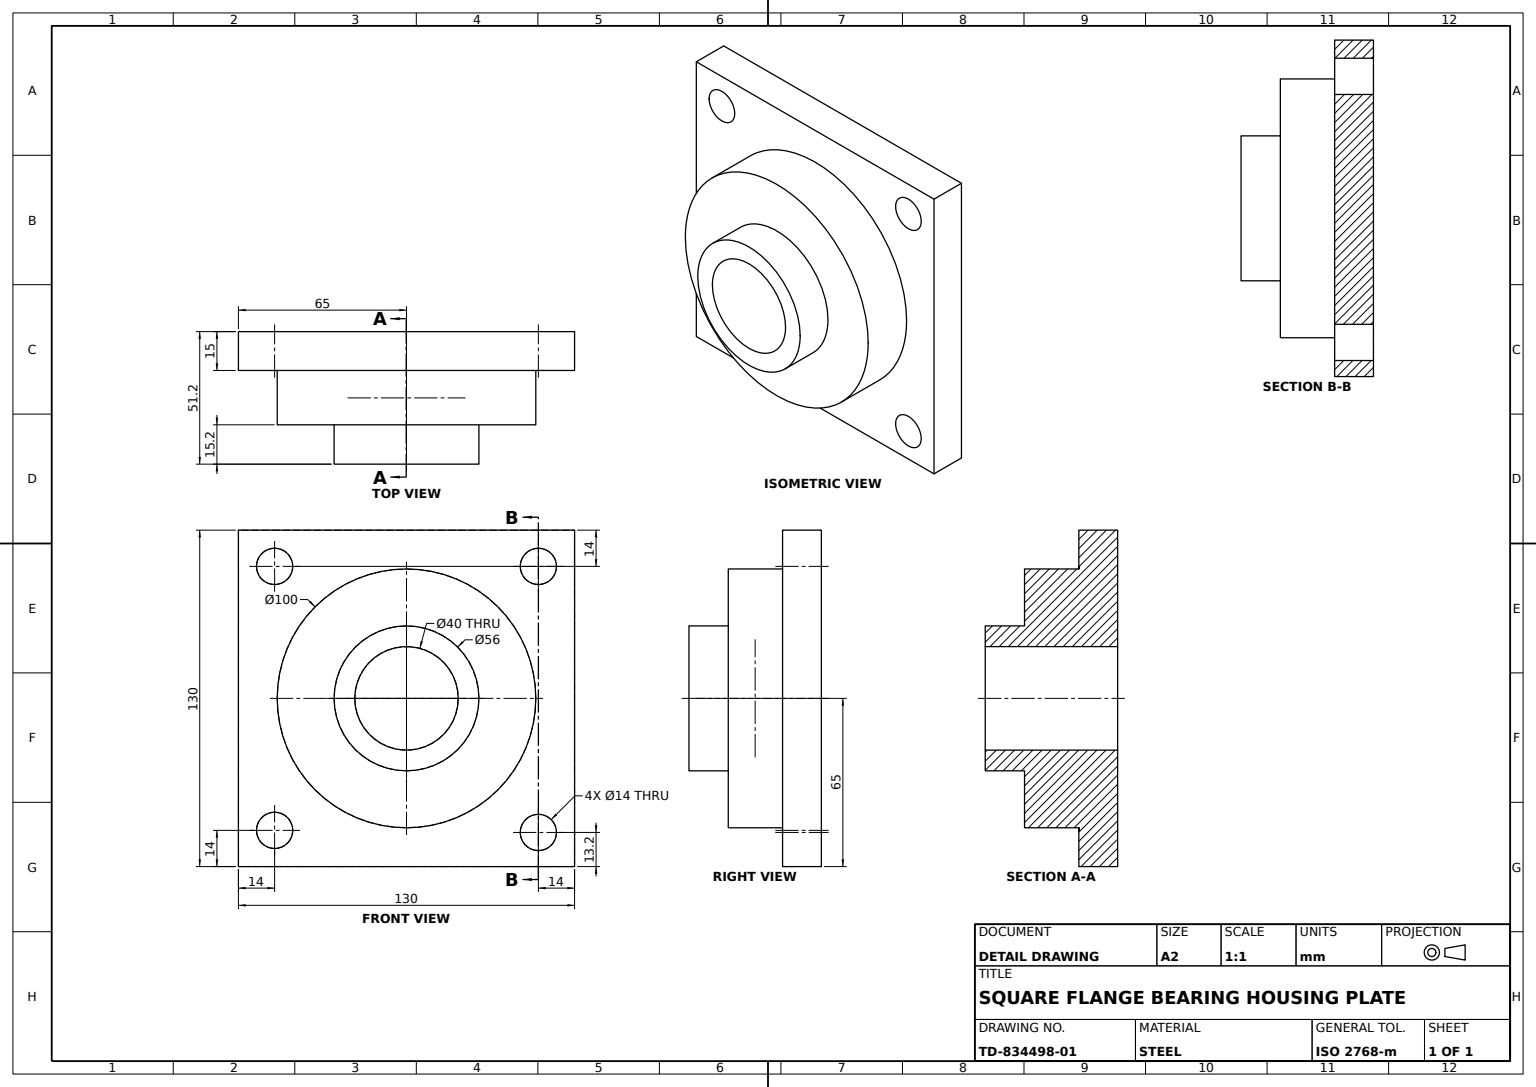
SolidWorks part; units mm, degrees
material "Plain Carbon Steel"
ref_plane "Front Plane" through (0, 0, 0) normal (0, 0, 1) x (1, 0, 0)
ref_plane "Top Plane" through (0, 0, 0) normal (0, 1, 0) x (1, 0, 0)
ref_plane "Right Plane" through (0, 0, 0) normal (1, 0, 0) x (0, 0, -1)
sketch "Flange Plate Sketch" plane through (0, 0, 0) normal (0, 0, 1) x (1, 0, 0)
  line L0 (0, 0) -> (130, 0)
  line L1 (130, 0) -> (130, 130)
  line L2 (130, 130) -> (0, 130)
  line L3 (0, 130) -> (0, 0)
  dimension "D1" = 130
extrude "Flange Plate 130x130x15" add sketch "Flange Plate Sketch" along normal blind 15
sketch "Hub Sketch Ø100" plane through (0, 0, 15) normal (0, 0, 1) x (1, 0, 0)
  line L0 (0, 130) -> (0, 0) construction
  line L1 (0, 0) -> (130, 0) construction
  circle A0 centre (65, 65) radius 50
  dimension "D1" = 100
  dimension "D2" = 100
  dimension "D3" = 65
  dimension "D4" = 65
extrude "Hub Ø100" add sketch "Hub Sketch Ø100" along normal blind 21
sketch "Spigot Sketch Ø56" plane through (0, 0, 36) normal (0, 0, 1) x (1, 0, 0)
  circle A0 centre (65, 65) radius 28
  dimension "D1" = 56
  dimension "D2" = 56
extrude "Spigot Ø56" add sketch "Spigot Sketch Ø56" along normal blind 15.2
sketch "Bore Sketch Ø40" plane through (0, 0, 51.2) normal (0, 0, 1) x (1, 0, 0)
  circle A0 centre (65, 65) radius 20
  dimension "D1" = 40
  dimension "D2" = 40
extrude "Bore Ø40" cut sketch "Bore Sketch Ø40" against normal blind 51.2
sketch "Mounting Holes Sketch" plane through (0, 0, 15) normal (0, 0, 1) x (1, 0, 0)
  line L0 (130, 130) -> (0, 130) construction
  line L1 (0, 130) -> (0, 0) construction
  line L2 (130, 0) -> (130, 130) construction
  line L3 (0, 0) -> (130, 0) construction
  circle A0 centre (116, 116) radius 7
  circle A1 centre (14, 116) radius 7
  circle A2 centre (14, 14) radius 7
  circle A3 centre (116, 13.1965) radius 7
  dimension "D1" = 14
  dimension "D3" = 14
  dimension "D7" = 14
  dimension "D8" = 14
  dimension "D11" = 14
  dimension "D2" = 14
  dimension "D4" = 14
  dimension "D5" = 14
  dimension "D6" = 14
  dimension "D9" = 14
  dimension "D10" = 14
  dimension "D12" = 13.1965
extrude "Mounting Holes 4xØ14" cut sketch "Mounting Holes Sketch" against normal blind 15
